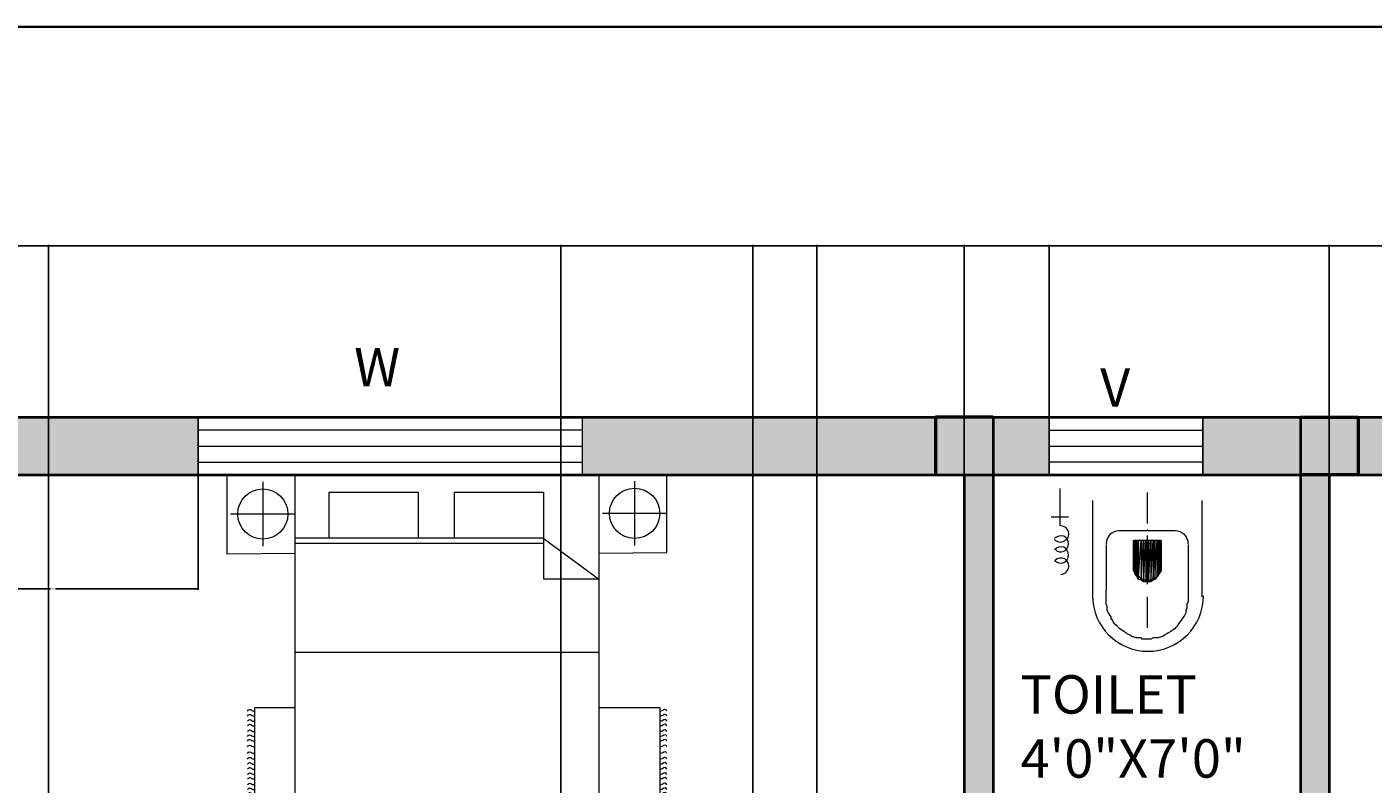
# Model space of a CAD drawing. Units: inches. Extents: x 25176543 to 25177243, y 80295576 to 80296086.
# Tile 4 of 11: x 25176668 to 25176879, y 80295968 to 80296086. Entities that reach past the tile are written whole.
import ezdxf

# ---------------------------------------------------------------- set-up
doc = ezdxf.new("R2010")
doc.units = ezdxf.units.IN
doc.header["$MEASUREMENT"] = 0
for name, color, linetype, lineweight in [('A-ANNO-DIMS', 2, 'Continuous', 18), ('A-ANNO-IDEN', 7, 'Continuous', 18), ('A-ANNO-TTLB', 7, 'Continuous', 35), ('A-AREA-IDEN', 7, 'Continuous', 18), ('A-COLS', 7, 'Continuous', 50), ('A-COLS-PATT', 251, 'Continuous', 13), ('A-FLOR-FIXT', 8, 'Continuous', 18), ('A-GLAZ', 4, 'Continuous', 18), ('A-WALL', 7, 'Continuous', 40), ('A-WALL-PATT', 146, 'Continuous', 13), ('furniture', 31, 'Continuous', 13)]:
    doc.layers.add(name, color=color, linetype=linetype, lineweight=lineweight)
doc.styles.get("Standard").update_dxf_attribs({"font": 'arial.ttf'})
doc.dimstyles.get("Standard").update_dxf_attribs({"dimtxt": 0.18, "dimasz": 0.18, "dimexe": 0.18, "dimexo": 0.0625, "dimgap": 0.09, "dimtad": 0, "dimtih": 1, "dimtoh": 1, "dimdec": 4, "dimzin": 0, "dimdsep": 46, "dimtxsty": 'Standard', "dimcen": 0.09, "dimadec": 0, "dimazin": 0, "dimtfac": 1, "dimtdec": 4, "dimtofl": 0, "dimtmove": 0, "dimatfit": 3, "dimfxl": 1, "dimtolj": 1, "dimtzin": 0, "dimarcsym": 0})

# ---------------------------------------------------------------- blocks, each defined once
blk = doc.blocks.new('BED-DOUBLE-WITH-NIGHTSTANDS')
for p, q in [((5.6, 61.62), (5.6, 51.56)), ((63.65, 61.72), (63.65, 51.66)), ((10.63, 56.59), (0.57, 56.59)), ((68.68, 56.69), (58.62, 56.69)), ((49.39, 52.82), (10.63, 52.82)), ((49.39, 52.82), (58, 46.47)), ((49.44, 52.82), (49.44, 46.47)), ((49.44, 52), (10.63, 52)), ((49.44, 46.47), (58, 46.47)), ((58.05, 34.96), (10.63, 34.96)), ((4.35, 0), (4.35, 26.37)), ((4.35, 26.37), (10.65, 26.37)), ((58.05, 26.37), (67.59, 26.37)), ((67.59, 26.37), (67.59, 0)), ((67.59, 0), (4.35, 0))]:
    blk.add_line(p, q)
for points in [[(0, 50.39), (10.63, 50.5), (10.63, 62.68), (0, 62.58)], [(58.05, 62.68), (58.05, 11.37), (10.63, 11.37), (10.63, 62.68)], [(58.05, 50.5), (68.68, 50.6), (68.68, 62.78), (58.05, 62.68)], [(29.88, 59.98), (29.88, 52.82), (15.98, 52.82), (15.98, 59.98)], [(49.44, 59.98), (49.44, 52.82), (35.55, 52.82), (35.55, 59.98)]]:
    blk.add_lwpolyline(points, close=True)
for centre in [(5.6, 56.59), (63.65, 56.69)]:
    blk.add_circle(centre, 3.92)
for points, knots in [([(3.23, 25.84), (3.32, 25.96), (3.52, 26.2), (3.86, 25.96), (4.14, 25.78), (4.29, 25.89), (4.35, 25.94)], [0, 0, 0, 0, 0.400747, 0.791423, 1.067667, 1.29709, 1.29709, 1.29709, 1.29709]), ([(3.23, 25.06), (3.32, 25.18), (3.52, 25.42), (3.86, 25.18), (4.14, 25.01), (4.29, 25.11), (4.35, 25.16)], [0, 0, 0, 0, 0.400747, 0.791423, 1.067667, 1.29709, 1.29709, 1.29709, 1.29709]), ([(68.71, 25.84), (68.61, 25.96), (68.42, 26.2), (68.08, 25.96), (67.8, 25.78), (67.65, 25.89), (67.58, 25.94)], [0, 0, 0, 0, 0.400747, 0.791423, 1.067667, 1.29709, 1.29709, 1.29709, 1.29709]), ([(68.71, 25.06), (68.61, 25.18), (68.42, 25.42), (68.08, 25.18), (67.8, 25.01), (67.65, 25.11), (67.58, 25.16)], [0, 0, 0, 0, 0.400747, 0.791423, 1.067667, 1.29709, 1.29709, 1.29709, 1.29709]), ([(3.23, 24.24), (3.32, 24.36), (3.52, 24.6), (3.86, 24.36), (4.14, 24.19), (4.29, 24.3), (4.35, 24.34)], [0, 0, 0, 0, 0.400747, 0.791423, 1.067667, 1.29709, 1.29709, 1.29709, 1.29709]), ([(3.23, 23.51), (3.32, 23.63), (3.52, 23.87), (3.86, 23.63), (4.14, 23.46), (4.29, 23.57), (4.35, 23.62)], [0, 0, 0, 0, 0.400747, 0.791423, 1.067667, 1.29709, 1.29709, 1.29709, 1.29709]), ([(68.71, 24.24), (68.61, 24.36), (68.42, 24.6), (68.08, 24.36), (67.8, 24.19), (67.65, 24.3), (67.58, 24.34)], [0, 0, 0, 0, 0.400747, 0.791423, 1.067667, 1.29709, 1.29709, 1.29709, 1.29709]), ([(68.71, 23.51), (68.61, 23.63), (68.42, 23.87), (68.08, 23.63), (67.8, 23.46), (67.65, 23.57), (67.58, 23.62)], [0, 0, 0, 0, 0.400747, 0.791423, 1.067667, 1.29709, 1.29709, 1.29709, 1.29709]), ([(3.23, 22.63), (3.32, 22.75), (3.52, 22.99), (3.86, 22.75), (4.14, 22.58), (4.29, 22.69), (4.35, 22.73)], [0, 0, 0, 0, 0.400747, 0.791423, 1.067667, 1.29709, 1.29709, 1.29709, 1.29709]), ([(3.23, 21.88), (3.32, 22), (3.52, 22.24), (3.86, 22), (4.14, 21.83), (4.29, 21.93), (4.35, 21.98)], [0, 0, 0, 0, 0.400747, 0.791423, 1.067667, 1.29709, 1.29709, 1.29709, 1.29709]), ([(3.23, 21.15), (3.32, 21.27), (3.52, 21.51), (3.86, 21.27), (4.14, 21.1), (4.29, 21.21), (4.35, 21.25)], [0, 0, 0, 0, 0.400747, 0.791423, 1.067667, 1.29709, 1.29709, 1.29709, 1.29709]), ([(68.71, 22.63), (68.61, 22.75), (68.42, 22.99), (68.08, 22.75), (67.8, 22.58), (67.65, 22.69), (67.58, 22.73)], [0, 0, 0, 0, 0.400747, 0.791423, 1.067667, 1.29709, 1.29709, 1.29709, 1.29709]), ([(68.71, 21.88), (68.61, 22), (68.42, 22.24), (68.08, 22), (67.8, 21.83), (67.65, 21.93), (67.58, 21.98)], [0, 0, 0, 0, 0.400747, 0.791423, 1.067667, 1.29709, 1.29709, 1.29709, 1.29709]), ([(68.71, 21.15), (68.61, 21.27), (68.42, 21.51), (68.08, 21.27), (67.8, 21.1), (67.65, 21.21), (67.58, 21.25)], [0, 0, 0, 0, 0.400747, 0.791423, 1.067667, 1.29709, 1.29709, 1.29709, 1.29709]), ([(3.23, 20.27), (3.32, 20.39), (3.52, 20.63), (3.86, 20.39), (4.14, 20.22), (4.29, 20.32), (4.35, 20.37)], [0, 0, 0, 0, 0.400747, 0.791423, 1.067667, 1.29709, 1.29709, 1.29709, 1.29709]), ([(3.23, 19.23), (3.32, 19.35), (3.52, 19.59), (3.86, 19.35), (4.14, 19.18), (4.29, 19.29), (4.35, 19.33)], [0, 0, 0, 0, 0.400747, 0.791423, 1.067667, 1.29709, 1.29709, 1.29709, 1.29709]), ([(68.71, 20.27), (68.61, 20.39), (68.42, 20.63), (68.08, 20.39), (67.8, 20.22), (67.65, 20.32), (67.58, 20.37)], [0, 0, 0, 0, 0.400747, 0.791423, 1.067667, 1.29709, 1.29709, 1.29709, 1.29709]), ([(68.71, 19.23), (68.61, 19.35), (68.42, 19.59), (68.08, 19.35), (67.8, 19.18), (67.65, 19.29), (67.58, 19.33)], [0, 0, 0, 0, 0.400747, 0.791423, 1.067667, 1.29709, 1.29709, 1.29709, 1.29709]), ([(3.23, 18.35), (3.32, 18.47), (3.52, 18.71), (3.86, 18.47), (4.14, 18.3), (4.29, 18.4), (4.35, 18.45)], [0, 0, 0, 0, 0.400747, 0.791423, 1.067667, 1.29709, 1.29709, 1.29709, 1.29709]), ([(3.23, 17.53), (3.32, 17.65), (3.52, 17.89), (3.86, 17.65), (4.14, 17.48), (4.29, 17.59), (4.35, 17.64)], [0, 0, 0, 0, 0.400747, 0.791423, 1.067667, 1.29709, 1.29709, 1.29709, 1.29709]), ([(3.23, 16.76), (3.32, 16.88), (3.52, 17.12), (3.86, 16.88), (4.14, 16.7), (4.29, 16.81), (4.35, 16.86)], [0, 0, 0, 0, 0.400747, 0.791423, 1.067667, 1.29709, 1.29709, 1.29709, 1.29709]), ([(68.71, 18.35), (68.61, 18.47), (68.42, 18.71), (68.08, 18.47), (67.8, 18.3), (67.65, 18.4), (67.58, 18.45)], [0, 0, 0, 0, 0.400747, 0.791423, 1.067667, 1.29709, 1.29709, 1.29709, 1.29709]), ([(68.71, 17.53), (68.61, 17.65), (68.42, 17.89), (68.08, 17.65), (67.8, 17.48), (67.65, 17.59), (67.58, 17.64)], [0, 0, 0, 0, 0.400747, 0.791423, 1.067667, 1.29709, 1.29709, 1.29709, 1.29709]), ([(68.71, 16.76), (68.61, 16.88), (68.42, 17.12), (68.08, 16.88), (67.8, 16.7), (67.65, 16.81), (67.58, 16.86)], [0, 0, 0, 0, 0.400747, 0.791423, 1.067667, 1.29709, 1.29709, 1.29709, 1.29709]), ([(3.23, 15.94), (3.32, 16.06), (3.52, 16.3), (3.86, 16.06), (4.14, 15.89), (4.29, 16), (4.35, 16.04)], [0, 0, 0, 0, 0.400747, 0.791423, 1.067667, 1.29709, 1.29709, 1.29709, 1.29709]), ([(3.23, 15.21), (3.32, 15.33), (3.52, 15.57), (3.86, 15.33), (4.14, 15.16), (4.29, 15.27), (4.35, 15.32)], [0, 0, 0, 0, 0.400747, 0.791423, 1.067667, 1.29709, 1.29709, 1.29709, 1.29709]), ([(68.71, 15.94), (68.61, 16.06), (68.42, 16.3), (68.08, 16.06), (67.8, 15.89), (67.65, 16), (67.58, 16.04)], [0, 0, 0, 0, 0.400747, 0.791423, 1.067667, 1.29709, 1.29709, 1.29709, 1.29709]), ([(68.71, 15.21), (68.61, 15.33), (68.42, 15.57), (68.08, 15.33), (67.8, 15.16), (67.65, 15.27), (67.58, 15.32)], [0, 0, 0, 0, 0.400747, 0.791423, 1.067667, 1.29709, 1.29709, 1.29709, 1.29709]), ([(3.23, 14.33), (3.32, 14.45), (3.52, 14.69), (3.86, 14.45), (4.14, 14.28), (4.29, 14.38), (4.35, 14.43)], [0, 0, 0, 0, 0.400747, 0.791423, 1.067667, 1.29709, 1.29709, 1.29709, 1.29709]), ([(3.23, 13.58), (3.32, 13.7), (3.52, 13.94), (3.86, 13.7), (4.14, 13.53), (4.29, 13.63), (4.35, 13.68)], [0, 0, 0, 0, 0.400747, 0.791423, 1.067667, 1.29709, 1.29709, 1.29709, 1.29709]), ([(3.23, 12.85), (3.32, 12.97), (3.52, 13.21), (3.86, 12.97), (4.14, 12.8), (4.29, 12.9), (4.35, 12.95)], [0, 0, 0, 0, 0.400747, 0.791423, 1.067667, 1.29709, 1.29709, 1.29709, 1.29709]), ([(68.71, 14.33), (68.61, 14.45), (68.42, 14.69), (68.08, 14.45), (67.8, 14.28), (67.65, 14.38), (67.58, 14.43)], [0, 0, 0, 0, 0.400747, 0.791423, 1.067667, 1.29709, 1.29709, 1.29709, 1.29709]), ([(68.71, 13.58), (68.61, 13.7), (68.42, 13.94), (68.08, 13.7), (67.8, 13.53), (67.65, 13.63), (67.58, 13.68)], [0, 0, 0, 0, 0.400747, 0.791423, 1.067667, 1.29709, 1.29709, 1.29709, 1.29709]), ([(68.71, 12.85), (68.61, 12.97), (68.42, 13.21), (68.08, 12.97), (67.8, 12.8), (67.65, 12.9), (67.58, 12.95)], [0, 0, 0, 0, 0.400747, 0.791423, 1.067667, 1.29709, 1.29709, 1.29709, 1.29709]), ([(3.23, 11.97), (3.32, 12.09), (3.52, 12.33), (3.86, 12.09), (4.14, 11.92), (4.29, 12.02), (4.35, 12.07)], [0, 0, 0, 0, 0.400747, 0.791423, 1.067667, 1.29709, 1.29709, 1.29709, 1.29709]), ([(3.23, 10.93), (3.32, 11.05), (3.52, 11.29), (3.86, 11.05), (4.14, 10.88), (4.29, 10.99), (4.35, 11.03)], [0, 0, 0, 0, 0.400747, 0.791423, 1.067667, 1.29709, 1.29709, 1.29709, 1.29709]), ([(68.71, 11.97), (68.61, 12.09), (68.42, 12.33), (68.08, 12.09), (67.8, 11.92), (67.65, 12.02), (67.58, 12.07)], [0, 0, 0, 0, 0.400747, 0.791423, 1.067667, 1.29709, 1.29709, 1.29709, 1.29709]), ([(68.71, 10.93), (68.61, 11.05), (68.42, 11.29), (68.08, 11.05), (67.8, 10.88), (67.65, 10.99), (67.58, 11.03)], [0, 0, 0, 0, 0.400747, 0.791423, 1.067667, 1.29709, 1.29709, 1.29709, 1.29709]), ([(3.23, 10.05), (3.32, 10.17), (3.52, 10.41), (3.86, 10.17), (4.14, 10), (4.29, 10.1), (4.35, 10.15)], [0, 0, 0, 0, 0.400747, 0.791423, 1.067667, 1.29709, 1.29709, 1.29709, 1.29709]), ([(3.23, 9.23), (3.32, 9.35), (3.52, 9.59), (3.86, 9.35), (4.14, 9.18), (4.29, 9.29), (4.35, 9.34)], [0, 0, 0, 0, 0.400747, 0.791423, 1.067667, 1.29709, 1.29709, 1.29709, 1.29709]), ([(3.23, 8.54), (3.32, 8.66), (3.52, 8.9), (3.86, 8.66), (4.14, 8.49), (4.29, 8.6), (4.35, 8.65)], [0, 0, 0, 0, 0.400747, 0.791423, 1.067667, 1.29709, 1.29709, 1.29709, 1.29709]), ([(68.71, 10.05), (68.61, 10.17), (68.42, 10.41), (68.08, 10.17), (67.8, 10), (67.65, 10.1), (67.58, 10.15)], [0, 0, 0, 0, 0.400747, 0.791423, 1.067667, 1.29709, 1.29709, 1.29709, 1.29709]), ([(68.71, 9.23), (68.61, 9.35), (68.42, 9.59), (68.08, 9.35), (67.8, 9.18), (67.65, 9.29), (67.58, 9.34)], [0, 0, 0, 0, 0.400747, 0.791423, 1.067667, 1.29709, 1.29709, 1.29709, 1.29709]), ([(68.71, 8.54), (68.61, 8.66), (68.42, 8.9), (68.08, 8.66), (67.8, 8.49), (67.65, 8.6), (67.58, 8.65)], [0, 0, 0, 0, 0.400747, 0.791423, 1.067667, 1.29709, 1.29709, 1.29709, 1.29709]), ([(3.23, 7.73), (3.32, 7.85), (3.52, 8.09), (3.86, 7.85), (4.14, 7.68), (4.29, 7.78), (4.35, 7.83)], [0, 0, 0, 0, 0.400747, 0.791423, 1.067667, 1.29709, 1.29709, 1.29709, 1.29709]), ([(3.23, 7), (3.32, 7.12), (3.52, 7.36), (3.86, 7.12), (4.14, 6.95), (4.29, 7.05), (4.35, 7.1)], [0, 0, 0, 0, 0.400747, 0.791423, 1.067667, 1.29709, 1.29709, 1.29709, 1.29709]), ([(3.23, 6.12), (3.32, 6.24), (3.52, 6.48), (3.86, 6.24), (4.14, 6.07), (4.29, 6.17), (4.35, 6.22)], [0, 0, 0, 0, 0.400747, 0.791423, 1.067667, 1.29709, 1.29709, 1.29709, 1.29709]), ([(68.71, 7.73), (68.61, 7.85), (68.42, 8.09), (68.08, 7.85), (67.8, 7.68), (67.65, 7.78), (67.58, 7.83)], [0, 0, 0, 0, 0.400747, 0.791423, 1.067667, 1.29709, 1.29709, 1.29709, 1.29709]), ([(68.71, 7), (68.61, 7.12), (68.42, 7.36), (68.08, 7.12), (67.8, 6.95), (67.65, 7.05), (67.58, 7.1)], [0, 0, 0, 0, 0.400747, 0.791423, 1.067667, 1.29709, 1.29709, 1.29709, 1.29709]), ([(68.71, 6.12), (68.61, 6.24), (68.42, 6.48), (68.08, 6.24), (67.8, 6.07), (67.65, 6.17), (67.58, 6.22)], [0, 0, 0, 0, 0.400747, 0.791423, 1.067667, 1.29709, 1.29709, 1.29709, 1.29709]), ([(3.23, 5.36), (3.32, 5.49), (3.52, 5.73), (3.86, 5.49), (4.14, 5.31), (4.29, 5.42), (4.35, 5.47)], [0, 0, 0, 0, 0.400747, 0.791423, 1.067667, 1.29709, 1.29709, 1.29709, 1.29709]), ([(3.23, 4.64), (3.32, 4.76), (3.52, 5), (3.86, 4.76), (4.14, 4.59), (4.29, 4.69), (4.35, 4.74)], [0, 0, 0, 0, 0.400747, 0.791423, 1.067667, 1.29709, 1.29709, 1.29709, 1.29709]), ([(68.71, 5.36), (68.61, 5.49), (68.42, 5.73), (68.08, 5.49), (67.8, 5.31), (67.65, 5.42), (67.58, 5.47)], [0, 0, 0, 0, 0.400747, 0.791423, 1.067667, 1.29709, 1.29709, 1.29709, 1.29709]), ([(68.71, 4.64), (68.61, 4.76), (68.42, 5), (68.08, 4.76), (67.8, 4.59), (67.66, 4.69), (67.59, 4.73)], [0, 0, 0, 0, 0.400747, 0.791423, 1.067667, 1.283686, 1.283686, 1.283686, 1.283686]), ([(3.23, 3.75), (3.32, 3.88), (3.52, 4.12), (3.86, 3.88), (4.14, 3.7), (4.29, 3.81), (4.35, 3.86)], [0, 0, 0, 0, 0.400747, 0.791423, 1.067667, 1.29709, 1.29709, 1.29709, 1.29709]), ([(3.23, 3.33), (3.32, 3.45), (3.52, 3.7), (3.86, 3.44), (4.14, 3.27), (4.29, 3.38), (4.35, 3.43)], [0, 0, 0, 0, 0.407265, 0.802015, 1.07826, 1.307683, 1.307683, 1.307683, 1.307683]), ([(3.23, 2.76), (3.32, 2.88), (3.52, 3.12), (3.86, 2.88), (4.14, 2.71), (4.29, 2.81), (4.35, 2.86)], [0, 0, 0, 0, 0.400747, 0.791423, 1.067667, 1.29709, 1.29709, 1.29709, 1.29709]), ([(3.23, 2.18), (3.32, 2.31), (3.52, 2.55), (3.86, 2.31), (4.14, 2.13), (4.29, 2.24), (4.35, 2.29)], [0, 0, 0, 0, 0.400747, 0.791423, 1.067667, 1.29709, 1.29709, 1.29709, 1.29709]), ([(3.23, 1.88), (3.32, 2), (3.52, 2.24), (3.86, 2), (4.14, 1.82), (4.29, 1.93), (4.35, 1.98)], [0, 0, 0, 0, 0.400747, 0.791423, 1.067667, 1.29709, 1.29709, 1.29709, 1.29709]), ([(68.71, 3.75), (68.61, 3.88), (68.42, 4.11), (68.08, 3.88), (67.8, 3.7), (67.66, 3.81), (67.59, 3.85)], [0, 0, 0, 0, 0.400747, 0.791423, 1.067667, 1.283686, 1.283686, 1.283686, 1.283686]), ([(68.71, 3.33), (68.61, 3.45), (68.42, 3.69), (68.08, 3.45), (67.8, 3.27), (67.66, 3.38), (67.59, 3.42)], [0, 0, 0, 0, 0.402903, 0.794912, 1.071156, 1.287177, 1.287177, 1.287177, 1.287177]), ([(68.71, 2.73), (68.61, 2.85), (68.42, 3.09), (68.08, 2.85), (67.8, 2.68), (67.66, 2.78), (67.59, 2.82)], [0, 0, 0, 0, 0.400747, 0.791423, 1.067667, 1.283686, 1.283686, 1.283686, 1.283686]), ([(68.71, 2.16), (68.61, 2.28), (68.42, 2.52), (68.08, 2.28), (67.8, 2.11), (67.66, 2.21), (67.59, 2.25)], [0, 0, 0, 0, 0.400747, 0.791423, 1.067667, 1.283686, 1.283686, 1.283686, 1.283686]), ([(68.71, 1.85), (68.61, 1.97), (68.42, 2.21), (68.08, 1.97), (67.8, 1.8), (67.66, 1.9), (67.59, 1.94)], [0, 0, 0, 0, 0.400747, 0.791423, 1.067667, 1.283686, 1.283686, 1.283686, 1.283686]), ([(3.23, 1.46), (3.32, 1.58), (3.52, 1.82), (3.86, 1.58), (4.14, 1.41), (4.29, 1.51), (4.35, 1.56)], [0, 0, 0, 0, 0.400747, 0.791423, 1.067667, 1.29709, 1.29709, 1.29709, 1.29709]), ([(3.23, 1.06), (3.32, 1.18), (3.52, 1.42), (3.86, 1.18), (4.14, 1.01), (4.29, 1.11), (4.35, 1.16)], [0, 0, 0, 0, 0.400747, 0.791423, 1.067667, 1.29709, 1.29709, 1.29709, 1.29709]), ([(3.23, 0.57), (3.32, 0.7), (3.52, 0.94), (3.86, 0.7), (4.14, 0.52), (4.29, 0.63), (4.35, 0.68)], [0, 0, 0, 0, 0.400747, 0.791423, 1.067667, 1.29709, 1.29709, 1.29709, 1.29709]), ([(3.23, 0.07), (3.32, 0.19), (3.52, 0.43), (3.86, 0.19), (4.14, 0.02), (4.29, 0.13), (4.35, 0.18)], [0, 0, 0, 0, 0.400747, 0.791423, 1.067667, 1.29709, 1.29709, 1.29709, 1.29709]), ([(68.71, 1.43), (68.61, 1.55), (68.42, 1.79), (68.08, 1.55), (67.8, 1.38), (67.65, 1.48), (67.58, 1.53)], [0, 0, 0, 0, 0.400747, 0.791423, 1.067667, 1.29709, 1.29709, 1.29709, 1.29709]), ([(68.71, 1.03), (68.61, 1.15), (68.42, 1.39), (68.08, 1.15), (67.8, 0.98), (67.65, 1.09), (67.58, 1.13)], [0, 0, 0, 0, 0.400747, 0.791423, 1.067667, 1.29709, 1.29709, 1.29709, 1.29709]), ([(68.71, 0.55), (68.61, 0.67), (68.42, 0.91), (68.08, 0.67), (67.8, 0.49), (67.65, 0.6), (67.58, 0.65)], [0, 0, 0, 0, 0.400747, 0.791423, 1.067667, 1.29709, 1.29709, 1.29709, 1.29709]), ([(68.71, 0.07), (68.61, 0.19), (68.42, 0.43), (68.08, 0.19), (67.8, 0.02), (67.65, 0.13), (67.58, 0.18)], [0, 0, 0, 0, 0.400747, 0.791423, 1.067667, 1.29709, 1.29709, 1.29709, 1.29709])]:
    blk.add_open_spline(points, degree=3, knots=knots)
blk = doc.blocks.new('WC-PLAN')
h = blk.add_hatch(color=256)
h.paths.add_polyline_path([(12.84, 17.3), (12.84, 12.59), (13.07, 17.3)])
h.paths.add_polyline_path([(12.84, 12.59), (13.07, 17.3), (13.07, 12.21)])
h = blk.add_hatch(color=256)
h.paths.add_polyline_path([(13.07, 17.3), (13.07, 12.21), (13.22, 17.3)])
h.paths.add_polyline_path([(13.07, 12.21), (13.22, 17.3), (13.22, 11.83)])
h = blk.add_hatch(color=256)
h.paths.add_polyline_path([(13.22, 17.3), (13.22, 11.83), (13.45, 17.3)])
h.paths.add_polyline_path([(13.22, 11.83), (13.45, 17.3), (13.45, 11.61)])
h = blk.add_hatch(color=256)
h.paths.add_polyline_path([(13.45, 17.3), (13.45, 11.61), (13.6, 17.3)])
h.paths.add_polyline_path([(13.45, 11.61), (13.6, 17.3), (13.6, 11.23)])
h = blk.add_hatch(color=256)
h.paths.add_polyline_path([(13.6, 17.3), (13.6, 11.23), (14.06, 17.3)])
h.paths.add_polyline_path([(13.6, 11.23), (14.06, 17.3), (14.06, 11.08)])
h = blk.add_hatch(color=256)
h.paths.add_polyline_path([(14.06, 17.3), (14.06, 11.08), (14.44, 17.3)])
h.paths.add_polyline_path([(14.06, 11.08), (14.44, 17.3), (14.44, 10.85)])
h = blk.add_hatch(color=256)
h.paths.add_polyline_path([(14.44, 17.3), (14.44, 10.85), (14.81, 17.3)])
h.paths.add_polyline_path([(14.44, 10.85), (14.81, 17.3), (14.81, 10.85)])
h = blk.add_hatch(color=256)
h.paths.add_polyline_path([(14.81, 17.3), (14.81, 10.85), (15.19, 17.3)])
h.paths.add_polyline_path([(14.81, 10.85), (15.19, 17.3), (15.19, 10.85)])
h = blk.add_hatch(color=256)
h.paths.add_polyline_path([(15.19, 17.3), (15.19, 10.85), (15.57, 17.3)])
h.paths.add_polyline_path([(15.19, 10.85), (15.57, 17.3), (15.57, 10.85)])
h = blk.add_hatch(color=256)
h.paths.add_polyline_path([(15.57, 17.3), (15.57, 10.85), (15.95, 17.3)])
h.paths.add_polyline_path([(15.57, 10.85), (15.95, 17.3), (15.95, 11.08)])
h = blk.add_hatch(color=256)
h.paths.add_polyline_path([(15.95, 17.3), (15.95, 11.08), (16.18, 17.3)])
h.paths.add_polyline_path([(15.95, 11.08), (16.18, 17.3), (16.18, 11.23)])
h = blk.add_hatch(color=256)
h.paths.add_polyline_path([(16.18, 17.3), (16.18, 11.23), (16.56, 17.3)])
h.paths.add_polyline_path([(16.18, 11.23), (16.56, 17.3), (16.56, 11.61)])
h = blk.add_hatch(color=256)
h.paths.add_polyline_path([(16.56, 17.3), (16.56, 11.61), (16.71, 17.3)])
h.paths.add_polyline_path([(16.56, 11.61), (16.71, 17.3), (16.71, 11.83)])
h = blk.add_hatch(color=256)
h.paths.add_polyline_path([(16.71, 17.3), (16.71, 11.83), (16.94, 17.3)])
h.paths.add_polyline_path([(16.71, 11.83), (16.94, 17.3), (16.94, 12.21)])
h = blk.add_hatch(color=256)
h.paths.add_polyline_path([(16.94, 17.3), (16.94, 12.21), (17.17, 17.3)])
h.paths.add_polyline_path([(16.94, 12.21), (17.17, 17.3), (17.17, 12.59)])
h.paths.add_polyline_path([(17.17, 17.3), (17.17, 12.59), (17.17, 12.97)])
for points in [[(1.37, 25.41), (1.37, 19.57), (1.37, 19.57)], [(6.47, 23.52), (6.47, 8.5), (6.47, 8.5)], [(14.97, 24.81), (14.97, 19.95), (14.97, 19.95)], [(23.54, 23.52), (23.54, 8.5), (23.54, 8.5)], [(2.73, 20.94), (0, 20.94), (0, 20.94)], [(14.97, 19.04), (15.04, 19.04), (15.04, 19.04)], [(19.29, 18.81), (10.57, 18.81), (10.57, 18.81)], [(17.17, 17.3), (12.84, 17.3), (12.84, 17.3)], [(12.84, 17.3), (12.84, 12.97), (12.84, 12.97)], [(14.59, 16.84), (14.59, 16.92), (14.59, 16.92)], [(14.97, 16.84), (14.81, 16.84), (14.59, 16.84)], [(14.97, 18.05), (14.97, 10.47), (14.97, 10.47)], [(14.97, 16.84), (15.04, 16.92), (15.04, 16.92)], [(15.42, 16.84), (15.19, 16.84), (14.97, 16.84)], [(15.42, 16.84), (15.42, 16.92), (15.42, 16.92)], [(17.17, 17.3), (17.17, 12.97), (17.17, 12.97)], [(8.59, 16.69), (8.59, 9.48), (8.59, 9.48)], [(21.41, 16.69), (21.41, 9.48), (21.41, 9.48)], [(21.41, 9.48), (21.41, 8.72), (21.41, 8.12), (21.41, 7.74), (21.19, 7.36), (21.19, 6.98), (21.19, 6.75), (21.04, 6.37), (21.04, 5.99), (20.81, 5.61), (20.66, 5.39), (20.43, 5.01), (20.28, 4.85), (20.05, 4.48), (19.82, 4.25), (19.67, 3.87), (19.44, 3.64), (19.29, 3.49), (18.91, 3.26), (18.68, 3.11), (18.3, 2.88), (18.08, 2.73), (17.7, 2.5), (17.32, 2.28), (17.17, 2.28), (16.71, 2.12), (16.33, 2.12), (15.95, 2.12), (15.57, 1.9), (14.97, 1.9), (14.21, 1.9), (14.06, 2.12), (13.6, 2.12), (13.22, 2.12), (12.84, 2.28), (12.69, 2.28), (12.31, 2.5), (11.86, 2.73), (11.7, 2.88), (11.33, 3.11), (11.1, 3.26), (10.72, 3.49), (10.57, 3.64), (10.34, 3.87), (9.96, 4.25), (9.73, 4.48), (9.58, 4.85), (9.35, 5.01), (9.35, 5.39), (9.2, 5.61), (8.97, 5.99), (8.75, 6.37), (8.75, 6.75), (8.75, 6.98), (8.59, 7.36), (8.59, 7.74), (8.59, 8.12), (8.59, 8.72), (8.59, 9.48)], [(14.97, 8.5), (14.97, 3.64), (14.97, 3.64)]]:
    blk.add_lwpolyline(points)
for points in [[(12.84, 17.3), (12.84, 12.97)], [(12.84, 12.97), (12.84, 17.3), (12.84, 12.59)], [(12.84, 17.3), (12.84, 12.59), (13.07, 17.3)], [(12.84, 12.59), (13.07, 17.3), (13.07, 12.21)], [(13.07, 17.3), (13.07, 12.21), (13.22, 17.3)], [(13.07, 12.21), (13.22, 17.3), (13.22, 11.83)], [(13.22, 17.3), (13.22, 11.83), (13.45, 17.3)], [(13.22, 11.83), (13.45, 17.3), (13.45, 11.61)], [(13.45, 17.3), (13.45, 11.61), (13.6, 17.3)], [(13.45, 11.61), (13.6, 17.3), (13.6, 11.23)], [(13.6, 17.3), (13.6, 11.23), (14.06, 17.3)], [(13.6, 11.23), (14.06, 17.3), (14.06, 11.08)], [(14.06, 17.3), (14.06, 11.08), (14.44, 17.3)], [(14.06, 11.08), (14.44, 17.3), (14.44, 10.85)], [(14.44, 17.3), (14.44, 10.85), (14.81, 17.3)], [(14.44, 10.85), (14.81, 17.3), (14.81, 10.85)], [(14.81, 17.3), (14.81, 10.85), (15.19, 17.3)], [(14.81, 10.85), (15.19, 17.3), (15.19, 10.85)], [(15.19, 17.3), (15.19, 10.85), (15.57, 17.3)], [(15.19, 10.85), (15.57, 17.3), (15.57, 10.85)], [(15.57, 17.3), (15.57, 10.85), (15.95, 17.3)], [(15.57, 10.85), (15.95, 17.3), (15.95, 11.08)], [(15.95, 17.3), (15.95, 11.08), (16.18, 17.3)], [(15.95, 11.08), (16.18, 17.3), (16.18, 11.23)], [(16.18, 17.3), (16.18, 11.23), (16.56, 17.3)], [(16.18, 11.23), (16.56, 17.3), (16.56, 11.61)], [(16.56, 17.3), (16.56, 11.61), (16.71, 17.3)], [(16.56, 11.61), (16.71, 17.3), (16.71, 11.83)], [(16.71, 17.3), (16.71, 11.83), (16.94, 17.3)], [(16.71, 11.83), (16.94, 17.3), (16.94, 12.21)], [(16.94, 17.3), (16.94, 12.21), (17.17, 17.3)], [(16.94, 12.21), (17.17, 17.3), (17.17, 12.59)], [(17.17, 17.3), (17.17, 12.59), (17.17, 12.97)], [(17.17, 12.59), (17.17, 17.3), (17.17, 17.3)]]:
    blk.add_lwpolyline(points, close=True)
for points, knots in [([(0.53, 17.45), (0.91, 17.07), (1.59, 16.92), (2.05, 17.22), (2.05, 17.22), (2.58, 17.52), (2.88, 18.05), (2.73, 18.66), (2.73, 18.66), (2.58, 19.19), (2.05, 19.57), (1.52, 19.57)], [0, 0, 0, 0, 0.083333, 0.083333, 0.083333, 0.083334, 0.166667, 0.166667, 0.166667, 0.166668, 1, 1, 1, 1]), ([(0.61, 15.93), (0.91, 15.55), (1.52, 15.4), (1.97, 15.63), (1.97, 15.63), (2.43, 15.78), (2.73, 16.31), (2.73, 16.76), (2.73, 16.76), (2.73, 17.3), (2.43, 17.75), (1.97, 17.98), (1.97, 17.98), (1.44, 18.13), (0.91, 17.98), (0.53, 17.6)], [0, 0, 0, 0, 0.0625, 0.0625, 0.0625, 0.062501, 0.125, 0.125, 0.125, 0.125001, 0.1875, 0.1875, 0.1875, 0.187501, 1, 1, 1, 1]), ([(0.53, 14.19), (0.91, 13.81), (1.44, 13.65), (1.97, 13.88), (1.97, 13.88), (2.43, 14.03), (2.73, 14.49), (2.73, 15.02), (2.73, 15.02), (2.73, 15.55), (2.43, 16.01), (1.97, 16.23), (1.97, 16.23), (1.44, 16.39), (0.91, 16.23), (0.53, 15.85)], [0, 0, 0, 0, 0.0625, 0.0625, 0.0625, 0.062501, 0.125, 0.125, 0.125, 0.125001, 0.1875, 0.1875, 0.1875, 0.187501, 1, 1, 1, 1]), ([(1.52, 11.99), (2.05, 11.99), (2.58, 12.44), (2.73, 12.97), (2.73, 12.97), (2.88, 13.5), (2.58, 14.11), (2.12, 14.41), (2.12, 14.41), (1.59, 14.64), (0.99, 14.56), (0.61, 14.19)], [0, 0, 0, 0, 0.083333, 0.083333, 0.083333, 0.083334, 0.166667, 0.166667, 0.166667, 0.166668, 1, 1, 1, 1]), ([(13.07, 13.12), (13.07, 11.99), (13.98, 11.08), (15.12, 11.08), (15.12, 11.08), (16.26, 11.08), (17.17, 11.99), (17.17, 13.12)], [0, 0, 0, 0, 0.125, 0.125, 0.125, 0.125001, 1, 1, 1, 1]), ([(6.47, 8.65), (6.47, 3.87), (10.34, 0), (15.12, 0), (15.12, 0), (19.9, 0), (23.77, 3.87), (23.77, 8.65)], [0, 0, 0, 0, 0.125, 0.125, 0.125, 0.125001, 1, 1, 1, 1])]:
    blk.add_open_spline(points, degree=3, knots=knots)
for points in [[(10.64, 18.81), (9.5, 18.81), (8.59, 17.9), (8.59, 16.76)], [(21.41, 16.76), (21.41, 17.9), (20.5, 18.81), (19.37, 18.81)]]:
    blk.add_open_spline(points, degree=3)
blk = doc.blocks.new('WIN-60IN')
for p, q in [((0, 9), (0, 0)), ((60, 9), (0, 9)), ((0, 9), (0, 4.5)), ((60, 0), (60, 9)), ((60, 7), (0, 7)), ((0, 4.5), (60, 4.5)), ((0, 2), (60, 2)), ((0, 0), (60, 0))]:
    blk.add_line(p, q)
blk = doc.blocks.new('VENT-WIN-24IN')
for p, q in [((0, 9), (0, 0)), ((0, 9), (24, 9)), ((24, 0), (24, 9)), ((0, 7), (24, 7)), ((0, 4.5), (24, 4.5)), ((24, 2), (0, 2)), ((0, 0), (24, 0))]:
    blk.add_line(p, q)
blk = doc.blocks.new('*D48')
at = {"layer": 'A-ANNO-DIMS', "color": 0, "lineweight": -2, "transparency": 16777216}
for p, q in [((25176625.3, 80295890.36), (25176625.3, 80296052.23)), ((25176625.48, 80296052.05), (25176875.16, 80296052.05)), ((25177125.62, 80296052.05), (25176875.95, 80296052.05)), ((25177125.8, 80296025.36), (25177125.8, 80296052.23))]:
    blk.add_line(p, q, dxfattribs=at)
at = {"layer": 'A-ANNO-DIMS', "color": 0, "transparency": 16777216}
for points in [[(25176625.48, 80296052.08), (25176625.48, 80296052.02), (25176625.3, 80296052.05)], [(25177125.62, 80296052.08), (25177125.62, 80296052.02), (25177125.8, 80296052.05)]]:
    blk.add_solid(points, dxfattribs=at)
at = {"layer": 'Defpoints', "color": 0, "transparency": 16777216}
for p in [(25177125.8, 80296052.05), (25177125.8, 80296025.3), (25176625.3, 80295890.3)]:
    blk.add_point(p, dxfattribs=at)
at = {"layer": 'A-ANNO-DIMS', "color": 0, "transparency": 16777216, "insert": (25176875.55, 80296052.05), "char_height": 0.18, "attachment_point": 5}
blk.add_mtext('\\A1;500.5', dxfattribs=at)
blk = doc.blocks.new('*D63')
at = {"layer": 'A-ANNO-DIMS', "color": 0, "lineweight": -2, "transparency": 16777216}
for p, q in [((25176649.8, 80296025.24), (25176649.8, 80295998.37)), ((25176695.19, 80296025.24), (25176695.19, 80295998.37)), ((25176649.98, 80295998.55), (25176672.1, 80295998.55)), ((25176695.01, 80295998.55), (25176672.89, 80295998.55))]:
    blk.add_line(p, q, dxfattribs=at)
at = {"layer": 'A-ANNO-DIMS', "color": 0, "transparency": 16777216}
for points in [[(25176649.98, 80295998.58), (25176649.98, 80295998.52), (25176649.8, 80295998.55)], [(25176695.01, 80295998.58), (25176695.01, 80295998.52), (25176695.19, 80295998.55)]]:
    blk.add_solid(points, dxfattribs=at)
at = {"layer": 'Defpoints', "color": 0, "transparency": 16777216}
for p in [(25176649.8, 80296025.3), (25176695.19, 80296025.3), (25176649.8, 80295998.55)]:
    blk.add_point(p, dxfattribs=at)
at = {"layer": 'A-ANNO-DIMS', "color": 0, "transparency": 16777216, "insert": (25176672.5, 80295998.55), "char_height": 0.18, "attachment_point": 5}
blk.add_mtext('\\A1;45.39', dxfattribs=at)
blk = doc.blocks.new('*D67')
at = {"layer": 'A-ANNO-DIMS', "color": 0, "lineweight": -2, "transparency": 16777216}
for p, q in [((25176814.8, 80296016.36), (25176814.8, 80296052.23)), ((25176814.98, 80296052.05), (25176821.04, 80296052.05)), ((25176827.86, 80296052.05), (25176821.81, 80296052.05)), ((25176828.04, 80296016.36), (25176828.04, 80296052.23))]:
    blk.add_line(p, q, dxfattribs=at)
at = {"layer": 'A-ANNO-DIMS', "color": 0, "transparency": 16777216}
for points in [[(25176814.98, 80296052.08), (25176814.98, 80296052.02), (25176814.8, 80296052.05)], [(25176827.86, 80296052.08), (25176827.86, 80296052.02), (25176828.04, 80296052.05)]]:
    blk.add_solid(points, dxfattribs=at)
at = {"layer": 'Defpoints', "color": 0, "transparency": 16777216}
for p in [(25176828.04, 80296052.05), (25176814.8, 80296016.3), (25176828.04, 80296016.3)]:
    blk.add_point(p, dxfattribs=at)
at = {"layer": 'A-ANNO-DIMS', "color": 0, "transparency": 16777216, "insert": (25176821.42, 80296052.05), "char_height": 0.18, "attachment_point": 5}
blk.add_mtext('\\A1;13.24', dxfattribs=at)
blk = doc.blocks.new('*D68')
at = {"layer": 'A-ANNO-DIMS', "color": 0, "lineweight": -2, "transparency": 16777216}
for p, q in [((25176871.8, 80296016.36), (25176871.8, 80296052.23)), ((25176871.98, 80296052.05), (25176878.04, 80296052.05)), ((25176885.01, 80296052.05), (25176878.95, 80296052.05)), ((25176885.19, 80296016.36), (25176885.19, 80296052.23))]:
    blk.add_line(p, q, dxfattribs=at)
at = {"layer": 'A-ANNO-DIMS', "color": 0, "transparency": 16777216}
for points in [[(25176871.98, 80296052.08), (25176871.98, 80296052.02), (25176871.8, 80296052.05)], [(25176885.01, 80296052.08), (25176885.01, 80296052.02), (25176885.19, 80296052.05)]]:
    blk.add_solid(points, dxfattribs=at)
at = {"layer": 'Defpoints', "color": 0, "transparency": 16777216}
for p in [(25176885.19, 80296052.05), (25176871.8, 80296016.3), (25176885.19, 80296016.3)]:
    blk.add_point(p, dxfattribs=at)
at = {"layer": 'A-ANNO-DIMS', "color": 0, "transparency": 16777216, "insert": (25176878.49, 80296052.05), "char_height": 0.18, "attachment_point": 5}
blk.add_mtext('\\A1;13.386', dxfattribs=at)
blk = doc.blocks.new('*D74')
at = {"layer": 'A-ANNO-DIMS', "color": 0, "lineweight": -2, "transparency": 16777216}
for p, q in [((25176671.8, 80295885.86), (25176671.8, 80296052.23)), ((25176671.98, 80296052.05), (25176711.58, 80296052.05)), ((25176751.62, 80296052.05), (25176712.02, 80296052.05)), ((25176751.8, 80295885.86), (25176751.8, 80296052.23))]:
    blk.add_line(p, q, dxfattribs=at)
at = {"layer": 'A-ANNO-DIMS', "color": 0, "transparency": 16777216}
for points in [[(25176671.98, 80296052.08), (25176671.98, 80296052.02), (25176671.8, 80296052.05)], [(25176751.62, 80296052.08), (25176751.62, 80296052.02), (25176751.8, 80296052.05)]]:
    blk.add_solid(points, dxfattribs=at)
at = {"layer": 'Defpoints', "color": 0, "transparency": 16777216}
for p in [(25176751.8, 80296052.05), (25176671.8, 80295885.8), (25176751.8, 80295885.8)]:
    blk.add_point(p, dxfattribs=at)
at = {"layer": 'A-ANNO-DIMS', "color": 0, "transparency": 16777216, "insert": (25176711.8, 80296052.05), "char_height": 0.18, "attachment_point": 5}
blk.add_mtext('\\A1;80', dxfattribs=at)
blk = doc.blocks.new('*D75')
at = {"layer": 'A-ANNO-DIMS', "color": 0, "lineweight": -2, "transparency": 16777216}
for p, q in [((25176781.8, 80295843.36), (25176781.8, 80296052.23)), ((25176781.98, 80296052.05), (25176786.59, 80296052.05)), ((25176791.62, 80296052.05), (25176787.01, 80296052.05)), ((25176791.8, 80295843.36), (25176791.8, 80296052.23))]:
    blk.add_line(p, q, dxfattribs=at)
at = {"layer": 'A-ANNO-DIMS', "color": 0, "transparency": 16777216}
for points in [[(25176781.98, 80296052.08), (25176781.98, 80296052.02), (25176781.8, 80296052.05)], [(25176791.62, 80296052.08), (25176791.62, 80296052.02), (25176791.8, 80296052.05)]]:
    blk.add_solid(points, dxfattribs=at)
at = {"layer": 'Defpoints', "color": 0, "transparency": 16777216}
for p in [(25176791.8, 80296052.05), (25176781.8, 80295843.3), (25176791.8, 80295843.3)]:
    blk.add_point(p, dxfattribs=at)
at = {"layer": 'A-ANNO-DIMS', "color": 0, "transparency": 16777216, "insert": (25176786.8, 80296052.05), "char_height": 0.18, "attachment_point": 5}
blk.add_mtext('\\A1;10', dxfattribs=at)

msp = doc.modelspace()

# ---------------------------------------------------------------- hatches: boundary and pattern name
at = {"layer": 'A-COLS-PATT'}
h = msp.add_hatch(color=256, dxfattribs=at)
h.dxf.hatch_style = 1
h.paths.add_polyline_path([(25176658.8016, 80296025.3022), (25176649.8016, 80296025.3022), (25176649.8016, 80296016.3022), (25176658.8016, 80296016.3022)])
h.paths.add_polyline_path([(25176819.3016, 80296025.3022), (25176810.3016, 80296025.3022), (25176810.3016, 80296016.3022), (25176819.3016, 80296016.3022)])
h.paths.add_polyline_path([(25176876.3016, 80296025.3022), (25176867.3016, 80296025.3022), (25176867.3016, 80296016.3022), (25176876.3016, 80296016.3022)])
h.paths.add_polyline_path([(25177013.3016, 80296025.3022), (25177004.3016, 80296025.3022), (25177004.3016, 80296016.3022), (25177013.3016, 80296016.3022)])
h.paths.add_polyline_path([(25176819.3016, 80295890.3022), (25176810.3016, 80295890.3022), (25176810.3016, 80295881.3022), (25176819.3016, 80295881.3022)])
h.paths.add_polyline_path([(25176658.8016, 80295890.3022), (25176649.8016, 80295890.3022), (25176649.8016, 80295881.3022), (25176658.8016, 80295881.3022)])
h.paths.add_polyline_path([(25177125.8016, 80296025.3022), (25177116.8016, 80296025.3022), (25177116.8016, 80296016.3022), (25177125.8016, 80296016.3022)])
h.paths.add_polyline_path([(25177125.8016, 80295848.3022), (25177116.8016, 80295848.3022), (25177116.8016, 80295839.3022), (25177125.8016, 80295839.3022)])
h.paths.add_polyline_path([(25177013.3016, 80295848.3022), (25177004.3016, 80295848.3022), (25177004.3016, 80295839.3022), (25177013.3016, 80295839.3022)])
h.paths.add_polyline_path([(25177125.8016, 80295676.8022), (25177116.8016, 80295676.8022), (25177116.8016, 80295667.8022), (25177125.8016, 80295667.8022)])
h.paths.add_polyline_path([(25177013.3016, 80295676.8022), (25177004.3016, 80295676.8022), (25177004.3016, 80295667.8022), (25177013.3016, 80295667.8022)])
h.paths.add_polyline_path([(25176842.3016, 80295676.8022), (25176833.3016, 80295676.8022), (25176833.3016, 80295667.8022), (25176842.3016, 80295667.8022)])
h.paths.add_polyline_path([(25176893.3016, 80295676.8022), (25176884.3016, 80295676.8022), (25176884.3016, 80295667.8022), (25176893.3016, 80295667.8022)])
h.paths.add_polyline_path([(25176842.3016, 80295807.3022), (25176833.3016, 80295807.3022), (25176833.3016, 80295798.3022), (25176842.3016, 80295798.3022)])
h.paths.add_polyline_path([(25176658.8016, 80295807.3022), (25176649.8016, 80295807.3022), (25176649.8016, 80295798.3022), (25176658.8016, 80295798.3022)])
h.paths.add_polyline_path([(25176658.8016, 80295676.8022), (25176649.8016, 80295676.8022), (25176649.8016, 80295667.8022), (25176658.8016, 80295667.8022)])
at = {"layer": 'A-WALL-PATT'}
h = msp.add_hatch(color=256, dxfattribs=at)
h.dxf.hatch_style = 1
h.paths.add_polyline_path([(25176695.189, 80296025.3022), (25176658.8016, 80296025.3022), (25176658.8016, 80296016.3022), (25176695.189, 80296016.3022)])
h.paths.add_polyline_path([(25176810.3016, 80296025.3022), (25176755.189, 80296025.3022), (25176755.189, 80296016.3022), (25176810.3016, 80296016.3022)])
h.paths.add_polyline_path([(25176819.3016, 80296016.3022), (25176814.8016, 80296016.3022), (25176814.8016, 80295965.3022), (25176819.3016, 80295965.3022)], flags=17)
h.paths.add_polyline_path([(25176828.0421, 80296025.3022), (25176819.3016, 80296025.3022), (25176819.3016, 80296016.3022), (25176828.0421, 80296016.3022)])
h.paths.add_polyline_path([(25176867.3016, 80296025.3022), (25176852.0421, 80296025.3022), (25176852.0421, 80296016.3022), (25176867.3016, 80296016.3022)])
h.paths.add_polyline_path([(25176885.1873, 80296025.3022), (25176876.3016, 80296025.3022), (25176876.3016, 80296016.3022), (25176885.1873, 80296016.3022)])
h.paths.add_polyline_path([(25176919.8016, 80296025.3022), (25176909.1873, 80296025.3022), (25176909.1873, 80296016.3022), (25176919.8016, 80296016.3022)])
h.paths.add_polyline_path([(25176924.3016, 80296016.3022), (25176919.8016, 80296016.3022), (25176919.8016, 80295890.3022), (25176904.8016, 80295890.3022), (25176904.8016, 80295885.8022), (25176967.3016, 80295885.8022), (25176967.3016, 80295890.3022), (25176924.3016, 80295890.3022)])
h.paths.add_polyline_path([(25176924.3016, 80296025.3022), (25176919.8016, 80296025.3022), (25176919.8016, 80296016.3022), (25176924.3016, 80296016.3022)])
h.paths.add_polyline_path([(25176938.7147, 80296025.3022), (25176924.3016, 80296025.3022), (25176924.3016, 80296016.3022), (25176938.7147, 80296016.3022)])
h.paths.add_polyline_path([(25176871.8016, 80296016.3022), (25176867.3016, 80296016.3022), (25176867.3016, 80295932.3022), (25176819.3016, 80295932.3022), (25176819.3016, 80295933.3022), (25176814.8016, 80295933.3022), (25176814.8016, 80295932.3022), (25176814.8016, 80295927.3022), (25176819.3016, 80295927.3022), (25176819.3016, 80295927.8022), (25176867.3016, 80295927.8022), (25176867.3016, 80295885.8022), (25176871.8016, 80295885.8022), (25176872.8016, 80295885.8022), (25176872.8016, 80295890.3022), (25176871.8016, 80295890.3022)])
h.paths.add_polyline_path([(25177004.3016, 80296025.3022), (25176986.7147, 80296025.3022), (25176986.7147, 80296016.3022), (25177004.3016, 80296016.3022)])
h.paths.add_polyline_path([(25177035.845, 80296025.3022), (25177013.3016, 80296025.3022), (25177013.3016, 80296016.3022), (25177035.845, 80296016.3022)])
h.paths.add_polyline_path([(25177008.8016, 80296016.3022), (25177004.3016, 80296016.3022), (25177004.3016, 80295890.3022), (25177003.3016, 80295890.3022), (25177003.3016, 80295885.8022), (25177004.3016, 80295885.8022), (25177004.3016, 80295885.3022), (25177008.8016, 80295885.3022)])
h.paths.add_polyline_path([(25177116.8016, 80296025.3022), (25177095.845, 80296025.3022), (25177095.845, 80296016.3022), (25177116.8016, 80296016.3022)])
h.paths.add_polyline_path([(25177125.8016, 80296016.3022), (25177116.8016, 80296016.3022), (25177116.8016, 80295971.1334), (25177121.3016, 80295971.1334), (25177125.8016, 80295971.1334)])
h.paths.add_polyline_path([(25177116.8016, 80295848.3022), (25177013.3016, 80295848.3022), (25177013.3016, 80295843.8022), (25177116.8016, 80295843.8022)])
h.paths.add_polyline_path([(25177125.8016, 80295911.1334), (25177116.8016, 80295911.1334), (25177116.8016, 80295848.3022), (25177125.8016, 80295848.3022)])
h.paths.add_polyline_path([(25177008.8016, 80295802.3022), (25177004.3016, 80295802.3022), (25177004.3016, 80295676.8022), (25177008.8016, 80295676.8022)])
h.paths.add_polyline_path([(25176658.8016, 80295705.5694), (25176649.8016, 80295705.5694), (25176649.8016, 80295676.8022), (25176658.8016, 80295676.8022)])
h.paths.add_polyline_path([(25176658.8016, 80295798.3022), (25176649.8016, 80295798.3022), (25176649.8016, 80295765.5694), (25176654.3016, 80295765.5694), (25176658.8016, 80295765.5694)])
h.paths.add_polyline_path([(25176833.3016, 80295807.3022), (25176658.8016, 80295807.3022), (25176658.8016, 80295802.8022), (25176833.3016, 80295802.8022)])
h.paths.add_polyline_path([(25176842.3016, 80295761.3022), (25176837.8016, 80295761.3022), (25176837.8016, 80295676.8022), (25176842.3016, 80295676.8022)])
h.paths.add_polyline_path([(25176649.8016, 80295807.3022), (25176629.8016, 80295807.3022), (25176629.8016, 80295885.8022), (25176649.8016, 80295885.8022), (25176649.8016, 80295890.3022), (25176625.3016, 80295890.3022), (25176625.3016, 80295802.8022), (25176649.8016, 80295802.8022)])
h.paths.add_polyline_path([(25176810.3016, 80295890.3022), (25176658.8016, 80295890.3022), (25176658.8016, 80295885.8022), (25176810.3016, 80295885.8022)])
h.paths.add_polyline_path([(25176658.8016, 80295922.9263), (25176649.8016, 80295922.9263), (25176649.8016, 80295890.3022), (25176658.8016, 80295890.3022)])
h.paths.add_polyline_path([(25176658.8016, 80296016.3022), (25176649.8016, 80296016.3022), (25176649.8016, 80295982.9263), (25176654.3016, 80295982.9263), (25176658.8016, 80295982.9263)])

# ---------------------------------------------------------------- linework, layer by layer
at = {"layer": 'A-ANNO-TTLB'}
msp.add_lwpolyline([(25176542.8973, 80296086.2335), (25177242.9194, 80296086.2335), (25177242.9194, 80295575.9501), (25176542.8973, 80295575.9501)], close=True, dxfattribs=at)
at = {"layer": 'A-COLS'}
for p, q in [((25176819.3016, 80296025.3022), (25176810.3016, 80296025.3022)), ((25176810.3016, 80296025.3022), (25176810.3016, 80296016.3022)), ((25176867.3016, 80296025.3022), (25176876.3016, 80296025.3022)), ((25176876.3016, 80296025.3022), (25176876.3016, 80296016.3022)), ((25176876.3016, 80296016.3022), (25176867.3016, 80296016.3022))]:
    msp.add_line(p, q, dxfattribs=at)
at = {"layer": 'A-GLAZ'}
for p, q in [((25176828.0421, 80296016.3022), (25176828.0421, 80296025.3022)), ((25176852.0421, 80296025.3022), (25176852.0421, 80296016.3022)), ((25176852.0421, 80296016.3022), (25176828.0421, 80296016.3022))]:
    msp.add_line(p, q, dxfattribs=at)
at = {"layer": 'A-WALL'}
for p, q in [((25176649.8016, 80296025.3022), (25177125.8016, 80296025.3022)), ((25176819.3016, 80296025.3022), (25176819.3016, 80295965.3022)), ((25176867.3016, 80296025.3022), (25176867.3016, 80295932.3022)), ((25176649.8016, 80296016.3022), (25177125.8016, 80296016.3022)), ((25176814.8016, 80296016.3022), (25176814.8016, 80295927.3022)), ((25176871.8016, 80296016.3022), (25176871.8016, 80295890.3022))]:
    msp.add_line(p, q, dxfattribs=at)

# ---------------------------------------------------------------- block references
at = {"layer": 'A-FLOR-FIXT'}
msp.add_blockref('WC-PLAN', (25176828.371, 80295988.781), dxfattribs=at)
at = {"layer": 'A-GLAZ'}
for name, p in [('WIN-60IN', (25176695.189, 80296016.302)), ('VENT-WIN-24IN', (25176828.042, 80296016.302))]:
    msp.add_blockref(name, p, dxfattribs=at)
at = {"layer": 'furniture'}
msp.add_blockref('BED-DOUBLE-WITH-NIGHTSTANDS', (25176699.678, 80295953.621), dxfattribs=at)

# ---------------------------------------------------------------- texts
at = {"layer": 'A-ANNO-IDEN', "char_height": 6, "attachment_point": 1}
for s, width, insert in [('W', 24.139595, (25176719.535, 80296036.1454)), ('V', 12.911449, (25176836.0094, 80296032.9682))]:
    msp.add_mtext_dynamic_manual_height_columns(s, width=width, gutter_width=1, heights=[0], dxfattribs=dict(at, insert=insert))
at = {"layer": 'A-AREA-IDEN', "insert": (25176823.5899, 80295985.0546), "char_height": 6, "attachment_point": 1}
msp.add_mtext_dynamic_manual_height_columns('TOILET\\P4\'0"X7\'0"', width=34.900641, gutter_width=1, heights=[0], dxfattribs=at)

# ---------------------------------------------------------------- dimensions: what is measured, and where the dimension line sits
at = {"layer": 'A-ANNO-DIMS'}
for base, p1, p2, override, picture, middle in [((25177125.8016, 80296052.0522), (25176625.3016, 80295890.3022), (25177125.8016, 80296025.3022), {"dimdec": 1, "dimlfac": 1, "dimrnd": 0, "dimzin": 0, "dimdsep": 46, "dimlunit": 2}, '*D48', (25176875.5516, 80296052.0522)), ((25176751.8016, 80296052.0522), (25176671.8016, 80295885.8022), (25176751.8016, 80295885.8022), {"dimdec": 0, "dimlfac": 1, "dimrnd": 0, "dimzin": 0, "dimdsep": 46, "dimlunit": 2}, '*D74', (25176711.8016, 80296052.0522)), ((25176791.8016, 80296052.0522), (25176781.8016, 80295843.3022), (25176791.8016, 80295843.3022), {"dimdec": 0, "dimlfac": 1, "dimrnd": 0, "dimzin": 0, "dimdsep": 46, "dimlunit": 2}, '*D75', (25176786.8016, 80296052.0522)), ((25176828.0421, 80296052.0522), (25176814.8016, 80296016.3022), (25176828.0421, 80296016.3022), {"dimdec": 2, "dimlfac": 1, "dimrnd": 0, "dimzin": 0, "dimdsep": 46, "dimlunit": 2}, '*D67', (25176821.4218, 80296052.0522)), ((25176885.1873, 80296052.0522), (25176871.8016, 80296016.3022), (25176885.1873, 80296016.3022), {"dimdec": 3, "dimlfac": 1, "dimrnd": 0, "dimzin": 0, "dimdsep": 46, "dimlunit": 2}, '*D68', (25176878.4944, 80296052.0522))]:
    dim = msp.add_linear_dim(base=base, p1=p1, p2=p2, dimstyle='Standard', override=override, dxfattribs=at)
    dim.commit()
    dim.dimension.update_dxf_attribs({"geometry": picture, "text_midpoint": middle})
dim = msp.add_linear_dim(base=(25176649.8016, 80295998.5522), p1=(25176695.189, 80296025.3022), p2=(25176649.8016, 80296025.3022), angle=180, dimstyle='Standard', override={"dimdec": 2, "dimlfac": 1, "dimrnd": 0, "dimzin": 0, "dimdsep": 46, "dimlunit": 2}, dxfattribs=at)
dim.commit()
dim.dimension.update_dxf_attribs({"geometry": '*D63', "text_midpoint": (25176672.4953, 80295998.5522)})

doc.saveas('drawing.dxf')
